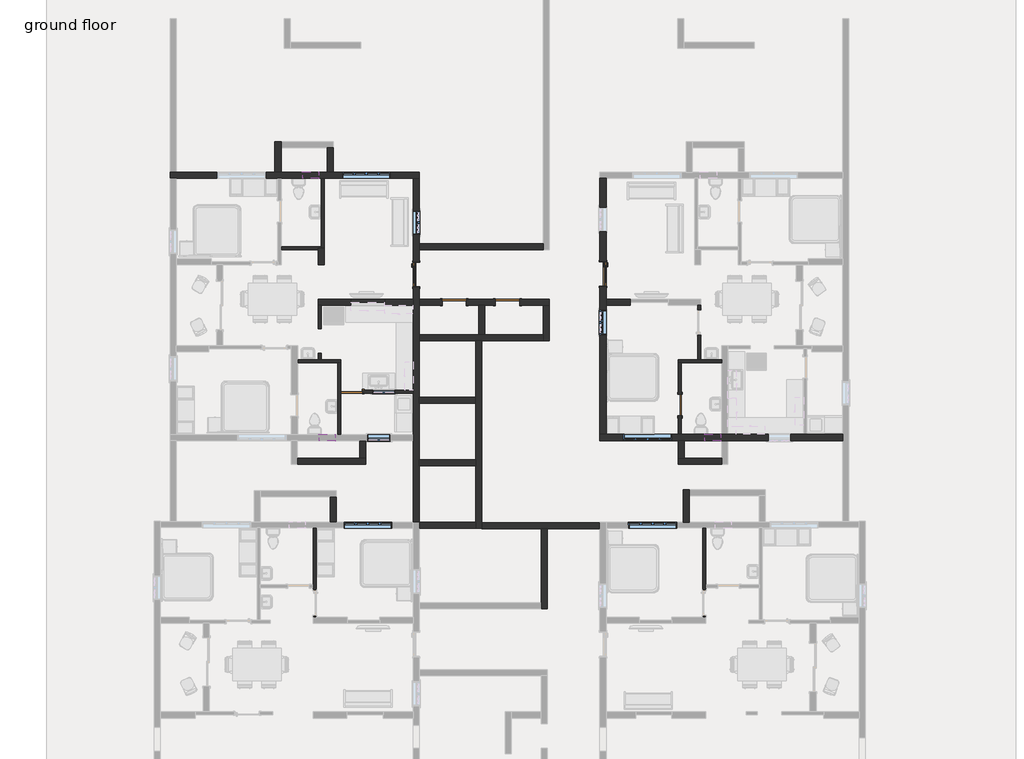
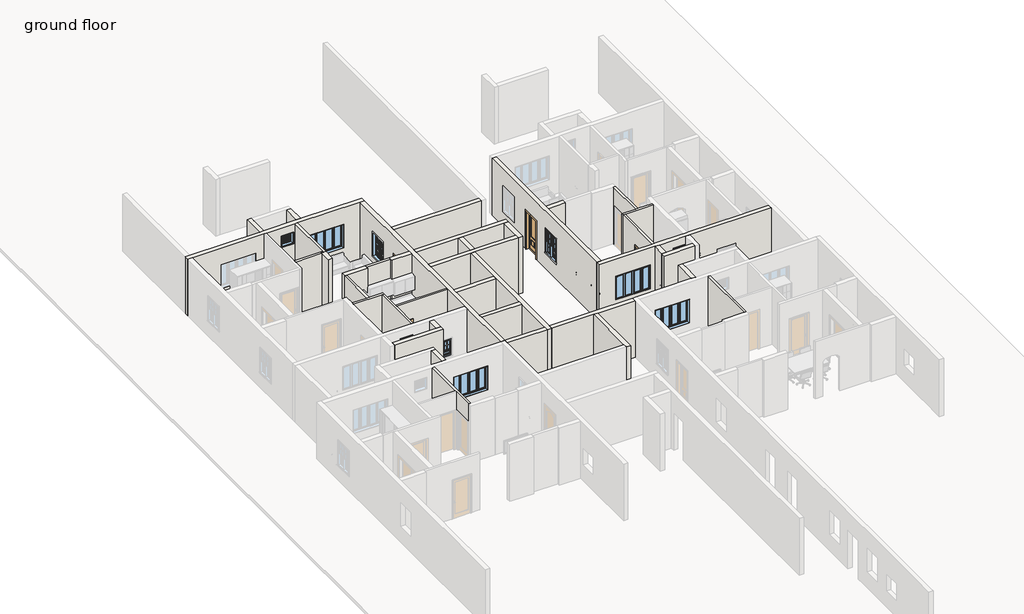
# One storey, part 5 of 16: 39 walls, 11 windows, 6 doors.
# Revit data of these elements (continued)
# Element 46 (IfcWindow, "Window-Casement-Double-Awning : 34\" x 36\"") (continued)
#   Interior Trim Visibility = yes
#   Exterior Trim Visibility = yes
#   Phase Created = New Construction
#   Materials on its faces: "Wood - Stained", "Glass", "Clad - White"
# Element 47 (IfcWindow, "Window-Casement-Double-Awning : 34\" x 36\"")
#   Mark = "88"
#   Window Inset = 0' - 0"
#   Interior Wall Closure = 0' - 2 1/4"
#   Frame Extension = 0' - 0 1/4"
#   Exterior Wall Closure = 0' - 1 1/4"
#   Interior Trim Visibility = yes
#   Exterior Trim Visibility = yes
#   Phase Created = New Construction
#   Materials on its faces: "Wood - Stained", "Glass", "Clad - White"
# Element 48 (IfcWindow, "Window-Casement-Multi-Sash-Horizontal : 72\" x 53\"")
#   Mark = "25"
#   Window Inset = 0' - 0 5/8"
#   Frame Gap 3 = 0' - 1 83/128"
#   Frame Gap 2 = 0' - 0 5/8"
#   Phase Created = New Construction
#   Materials on its faces: "Metal - Aluminum", "Glass"
# Element 49 (IfcWindow, "Window-Casement-Multi-Sash-Horizontal : 72\" x 53\"")
#   Mark = "26"
#   Window Inset = 0' - 0 5/8"
#   Frame Gap 3 = 0' - 1 83/128"
#   Frame Gap 2 = 0' - 0 5/8"
#   Phase Created = New Construction
#   Materials on its faces: "Metal - Aluminum", "Glass"
# Element 50 (IfcWindow, "Window-Casement-Multi-Sash-Horizontal : 72\" x 53\"")
#   Mark = "36"
#   Window Inset = 0' - 0 5/8"
#   Frame Gap 3 = 0' - 1 83/128"
#   Frame Gap 2 = 0' - 0 5/8"
#   Phase Created = New Construction
#   Materials on its faces: "Metal - Aluminum", "Glass"
# Element 51 (IfcWindow, "Window-Casement-Multi-Sash-Horizontal : 72\" x 53\"")
#   Mark = "39"
#   Window Inset = 0' - 0 5/8"
#   Frame Gap 3 = 0' - 1 83/128"
#   Frame Gap 2 = 0' - 0 5/8"
#   Phase Created = New Construction
#   Materials on its faces: "Metal - Aluminum", "Glass"
# Element 52 (IfcWindow, "Window-Louvers : 24\" x 24\"")
#   Mark = "97"
#   Blade Width = 1' - 10 1/2"
#   Phase Created = New Construction
#   Materials on its faces: "Birch"
# Element 53 (IfcWindow, "Window-Louvers : 24\" x 24\"")
#   Mark = "108"
#   Blade Width = 1' - 10 1/2"
#   Phase Created = New Construction
#   Materials on its faces: "Birch"
# Element 54 (IfcWindow, "Window-Louvers : 24\" x 24\"")
#   Mark = "109"
#   Blade Width = 1' - 10 1/2"
#   Phase Created = New Construction
#   Materials on its faces: "Birch"
# Element 55 (IfcWindow, "Window-Single-Hung-Double : 36\" x 52\"")
#   Mark = "49"
#   Window Inset = 0' - 0"
#   Interior Wall Closure = 0' - 1 1/2"
#   Frame Extension = 0' - 1 1/4"
#   Exterior Wall Closure = 0' - 0 1/2"
#   Interior Trim Visibility = yes
#   Indicator Visibility = yes
#   Exterior Trim Visibility = yes
#   Phase Created = New Construction
#   Materials on its faces: "Wood - Stained", "Glass", "Clad - White"
# Element 56 (IfcWindow, "Window-Single-Hung-Double : 36\" x 52\"")
#   Mark = "62"
#   Window Inset = 0' - 0"
#   Interior Wall Closure = 0' - 1 1/2"
#   Frame Extension = 0' - 1 1/4"
#   Exterior Wall Closure = 0' - 0 1/2"
#   Interior Trim Visibility = yes
#   Indicator Visibility = yes
#   Exterior Trim Visibility = yes
#   Phase Created = New Construction
#   Materials on its faces: "Wood - Stained", "Glass", "Clad - White"
# Materials
#   "Cherry": class "Wood", colour RGB 226 177 128, transparency 0, Description = "Prunus Serotina", Cost = 0
#   "Glass": class "Glass", colour RGB 0 128 192, transparency 0.75, Description = "Soda Lime Glass", Cost = 0
#   "Aluminum": class "Metal", colour RGB 247 247 247, transparency 0, Description = "Aluminum 6061", Cost = 0
#   "Door - Panel": class "Wood", colour RGB 210 159 95, transparency 0, Cost = 0
#   "Door - Frame": colour RGB 118 70 51, transparency 0, Cost = 0
#   "Wood - Stained": class "Wood", colour RGB 224 178 126, transparency 0, Cost = 0
#   "Clad - White": class "Wood", colour RGB 242 242 238, transparency 0, Cost = 0
#   "Metal - Aluminum": class "Metal", colour RGB 247 247 247, transparency 0
#   "Birch": class "Wood", colour RGB 224 178 126, transparency 0, Description = "Betula Alleghaniensis", Cost = 0
#   "Default Wall": colour RGB 128 128 128, transparency 0, Cost = 0
